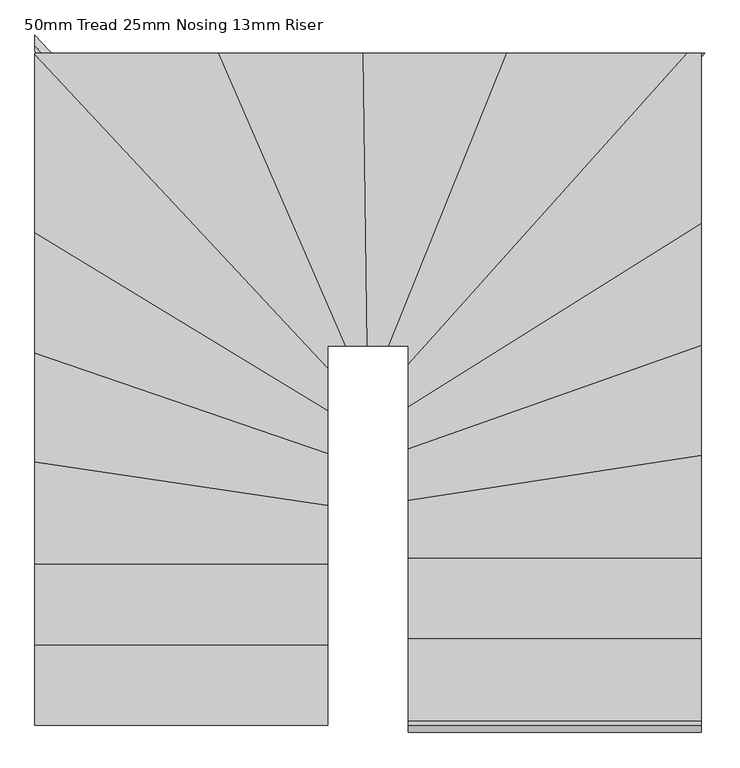
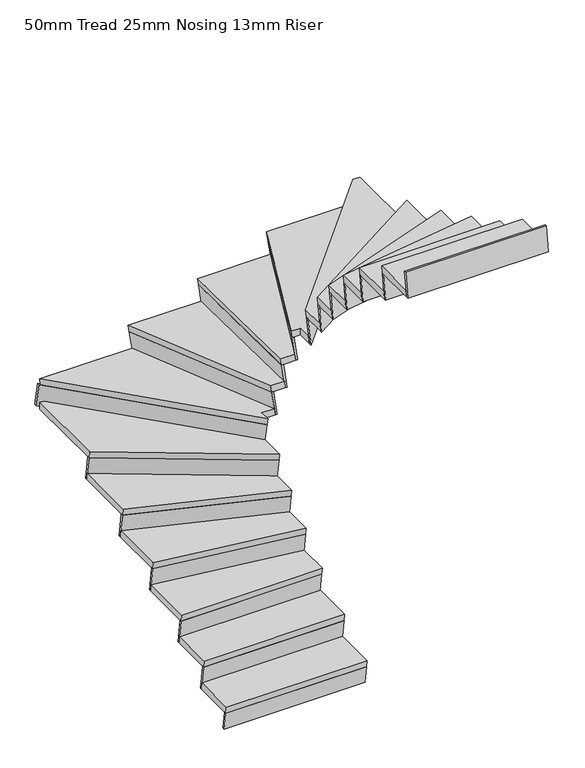
"""IFC4 building model written with IfcOpenShell, lengths in millimetres: stair flight geometry, 50mm Tread 25mm Nosing 13mm Riser."""

from ifc_helpers import new_model, si_unit, origin, place, context, project, spatial, faceted_brep, source, transform, mapped, element, save


def stair_flight_50mm_tread_25mm_nosing_13mm_riser_620a4597(model_context):
    return source(origin(), model_context, "Body", "Brep", [
        faceted_brep([(10289.7497541, -1105.5848061, 3227.2941176), (10289.7497541, -1098.6130213, 3177.2941176), (9289.7239729, -1098.6130213, 3177.2941176), (9289.7239729, -1105.5848061, 3227.2941176), (9289.7239729, -1405.5848061, 3227.2941176), (10289.7497541, -1405.5848061, 3227.2941176), (10289.7497541, -1398.6130213, 3177.2941176), (9289.7239729, -1398.6130213, 3177.2941176)], [[[0, 1, 2, 3]], [[3, 4, 5, 0]], [[2, 1, 6, 7]], [[4, 3, 2, 7]], [[0, 5, 6, 1]], [[5, 4, 7, 6]]]),
        faceted_brep([(10289.7497541, -1398.6130213, 3177.2941176), (10289.7497541, -1380.5848061, 3048.0), (10289.7497541, -1367.9638766, 3048.0), (10289.7497541, -1385.9920918, 3177.2941176), (9289.7239729, -1398.6130213, 3177.2941176), (9289.7239729, -1385.9920918, 3177.2941176), (9289.7239729, -1367.9638766, 3048.0), (9289.7239729, -1380.5848061, 3048.0)], [[[0, 1, 2, 3]], [[4, 5, 6, 7]], [[1, 0, 4, 7]], [[2, 1, 7, 6]], [[3, 2, 6, 5]], [[0, 3, 5, 4]]]),
        faceted_brep([(10289.7497541, -1123.6130213, 3356.5882353), (10289.7497541, -1098.6130213, 3177.2941176), (10289.7497541, -1085.9920918, 3177.2941176), (10289.7497541, -1110.9920918, 3356.5882353), (9289.7239729, -1123.6130213, 3356.5882353), (9289.7239729, -1110.9920918, 3356.5882353), (9289.7239729, -1085.9920918, 3177.2941176), (9289.7239729, -1098.6130213, 3177.2941176)], [[[0, 1, 2, 3]], [[4, 5, 6, 7]], [[1, 0, 4, 7]], [[2, 1, 7, 6]], [[3, 2, 6, 5]], [[0, 3, 5, 4]]]),
        faceted_brep([(9289.7239729, -830.5848061, 3406.5882353), (9289.7239729, -1130.5848061, 3406.5882353), (10289.7497541, -1130.5848061, 3406.5882353), (10289.7497541, -830.5848061, 3406.5882353), (9289.7239729, -823.6130213, 3356.5882353), (10289.7497541, -823.6130213, 3356.5882353), (10289.7497541, -1123.6130213, 3356.5882353), (9289.7239729, -1123.6130213, 3356.5882353)], [[[0, 1, 2, 3]], [[4, 5, 6, 7]], [[1, 0, 4, 7]], [[3, 2, 6, 5]], [[3, 5, 4, 0]], [[2, 1, 7, 6]]]),
        faceted_brep([(10289.7497541, -848.6130213, 3535.8823529), (10289.7497541, -823.6130213, 3356.5882353), (10289.7497541, -810.9920918, 3356.5882353), (10289.7497541, -835.9920918, 3535.8823529), (9289.7239729, -848.6130213, 3535.8823529), (9289.7239729, -835.9920918, 3535.8823529), (9289.7239729, -810.9920918, 3356.5882353), (9289.7239729, -823.6130213, 3356.5882353)], [[[0, 1, 2, 3]], [[4, 5, 6, 7]], [[1, 0, 4, 7]], [[2, 1, 7, 6]], [[3, 2, 6, 5]], [[0, 3, 5, 4]]]),
        faceted_brep([(9289.7239729, -480.7581684, 3585.8823529), (9289.7239729, -855.5848061, 3585.8823529), (10289.7497541, -855.5848061, 3585.8823529), (10289.7497541, -629.8587526, 3585.8823529), (9289.7239729, -473.7093187, 3535.8823529), (10289.7497541, -622.8099029, 3535.8823529), (10289.7497541, -848.6130213, 3535.8823529), (9289.7239729, -848.6130213, 3535.8823529)], [[[0, 1, 2, 3]], [[4, 5, 6, 7]], [[1, 0, 4, 7]], [[3, 2, 6, 5]], [[3, 5, 4, 0]], [[2, 1, 7, 6]]]),
        faceted_brep([(10289.7497541, -648.0862485, 3715.1764706), (10289.7497541, -622.8099029, 3535.8823529), (10289.7497541, -610.0494638, 3535.8823529), (10289.7497541, -635.3258095, 3715.1764706), (9289.7239729, -498.9856643, 3715.1764706), (9289.7239729, -486.2252253, 3715.1764706), (9289.7239729, -460.9488796, 3535.8823529), (9289.7239729, -473.7093187, 3535.8823529)], [[[0, 1, 2, 3]], [[4, 5, 6, 7]], [[1, 0, 4, 7]], [[2, 1, 7, 6]], [[3, 2, 6, 5]], [[0, 3, 5, 4]]]),
        faceted_brep([(9289.7239729, -107.774321, 3765.1764706), (9289.7239729, -506.034514, 3765.1764706), (10289.7497541, -655.1350982, 3765.1764706), (10289.7497541, -450.5397782, 3765.1764706), (9289.7239729, -100.4043758, 3715.1764706), (10289.7497541, -443.169833, 3715.1764706), (10289.7497541, -648.0862485, 3715.1764706), (9289.7239729, -498.9856643, 3715.1764706)], [[[0, 1, 2, 3]], [[4, 5, 6, 7]], [[1, 0, 4, 7]], [[3, 2, 6, 5]], [[3, 5, 4, 0]], [[2, 1, 7, 6]]]),
        faceted_brep([(10289.7497541, -469.5975895, 3894.4705882), (10289.7497541, -443.169833, 3715.1764706), (10289.7497541, -429.8281189, 3715.1764706), (10289.7497541, -456.2558754, 3894.4705882), (9289.7239729, -126.8321323, 3894.4705882), (9289.7239729, -113.4904182, 3894.4705882), (9289.7239729, -87.0626618, 3715.1764706), (9289.7239729, -100.4043758, 3715.1764706)], [[[0, 1, 2, 3]], [[4, 5, 6, 7]], [[1, 0, 4, 7]], [[2, 1, 7, 6]], [[3, 2, 6, 5]], [[0, 3, 5, 4]]]),
        faceted_brep([(9289.7239729, 306.1026023, 3944.4705882), (9289.7239729, -134.2020775, 3944.4705882), (10289.7497541, -476.9675347, 3944.4705882), (10289.7497541, -301.16869, 3944.4705882), (9289.7239729, 314.2591716, 3894.4705882), (10289.7497541, -293.0121207, 3894.4705882), (10289.7497541, -469.5975895, 3894.4705882), (9289.7239729, -126.8321323, 3894.4705882)], [[[0, 1, 2, 3]], [[4, 5, 6, 7]], [[1, 0, 4, 7]], [[3, 2, 6, 5]], [[3, 5, 4, 0]], [[2, 1, 7, 6]]]),
        faceted_brep([(10289.7497541, -322.2606186, 4073.7647059), (10289.7497541, -293.0121207, 3894.4705882), (10289.7497541, -278.2463915, 3894.4705882), (10289.7497541, -307.4948894, 4073.7647059), (9289.7239729, 285.0106737, 4073.7647059), (9289.7239729, 299.7764029, 4073.7647059), (9289.7239729, 329.0249008, 3894.4705882), (9289.7239729, 314.2591716, 3894.4705882)], [[[0, 1, 2, 3]], [[4, 5, 6, 7]], [[1, 0, 4, 7]], [[2, 1, 7, 6]], [[3, 2, 6, 5]], [[0, 3, 5, 4]]]),
        faceted_brep([(9320.7227269, 889.7143644, 4123.7647059), (9289.7239729, 889.7143644, 4123.7647059), (9289.7239729, 276.8541044, 4123.7647059), (10289.7497541, -330.4171879, 4123.7647059), (10289.7497541, -148.9817857, 4123.7647059), (9330.2573955, 889.7143644, 4073.7647059), (10289.7497541, -138.761613, 4073.7647059), (10289.7497541, -322.2606186, 4073.7647059), (9289.7239729, 285.0106737, 4073.7647059), (9289.7239729, 889.7143644, 4073.7647059)], [[[0, 1, 2, 3, 4]], [[5, 6, 7, 8, 9]], [[1, 0, 5, 9]], [[4, 3, 7, 6]], [[4, 6, 5, 0]], [[3, 2, 8, 7]], [[2, 1, 9, 8]]]),
        faceted_brep([(10289.7497541, -175.4099498, 4253.0588235), (10289.7497541, -138.761613, 4073.7647059), (10289.7497541, -120.2601701, 4073.7647059), (10289.7497541, -156.9085068, 4253.0588235), (9289.7239729, 896.5136394, 4253.0588235), (9289.7239729, 915.0150824, 4253.0588235), (9289.7239729, 951.6634191, 4073.7647059), (9289.7239729, 933.1619761, 4073.7647059)], [[[0, 1, 2, 3]], [[4, 5, 6, 7]], [[1, 0, 4, 7]], [[2, 1, 7, 6]], [[3, 2, 6, 5]], [[0, 3, 5, 4]]]),
        faceted_brep([(9944.3142793, 889.7143644, 4303.0588235), (9289.7239729, 889.7143644, 4303.0588235), (9289.7239729, 886.2934667, 4303.0588235), (10289.7497541, -185.6301224, 4303.0588235), (10289.7497541, -110.3114169, 4303.0588235), (10378.5813525, -110.3114169, 4303.0588235), (9951.9150537, 889.7143644, 4253.0588235), (10386.182127, -110.3114169, 4253.0588235), (10289.7497541, -110.3114169, 4253.0588235), (10289.7497541, -175.4099498, 4253.0588235), (9296.0671958, 889.7143644, 4253.0588235), (9289.7239729, 889.7143644, 4286.3228165)], [[[0, 1, 2, 3, 4, 5]], [[6, 7, 8, 9, 10]], [[1, 0, 6, 10, 11]], [[2, 1, 11]], [[4, 3, 9, 8]], [[5, 4, 8, 7]], [[5, 7, 6, 0]], [[3, 2, 11, 10, 9]]]),
        faceted_brep([(10358.9266439, -110.3114169, 4432.3529412), (10386.182127, -110.3114169, 4253.0588235), (10399.9417081, -110.3114169, 4253.0588235), (10372.6862251, -110.3114169, 4432.3529412), (9924.6595707, 889.7143644, 4432.3529412), (9938.4191519, 889.7143644, 4432.3529412), (9965.6746349, 889.7143644, 4253.0588235), (9951.9150537, 889.7143644, 4253.0588235)], [[[0, 1, 2, 3]], [[4, 5, 6, 7]], [[1, 0, 4, 7]], [[2, 1, 7, 6]], [[3, 2, 6, 5]], [[0, 3, 5, 4]]]),
        faceted_brep([(10435.8300538, 889.7143644, 4482.3529412), (9917.0587962, 889.7143644, 4482.3529412), (10351.3258695, -110.3114169, 4482.3529412), (10449.7733926, -110.3114169, 4482.3529412), (10442.8025162, 889.7143644, 4432.3529412), (10456.745855, -110.3114169, 4432.3529412), (10358.9266439, -110.3114169, 4432.3529412), (9924.6595707, 889.7143644, 4432.3529412)], [[[0, 1, 2, 3]], [[4, 5, 6, 7]], [[1, 0, 4, 7]], [[3, 2, 6, 5]], [[3, 5, 4, 0]], [[2, 1, 7, 6]]]),
        faceted_brep([(10431.7434251, -110.3114169, 4611.6470588), (10456.745855, -110.3114169, 4432.3529412), (10469.3680113, -110.3114169, 4432.3529412), (10444.3655813, -110.3114169, 4611.6470588), (10417.8000863, 889.7143644, 4611.6470588), (10430.4222425, 889.7143644, 4611.6470588), (10455.4246725, 889.7143644, 4432.3529412), (10442.8025162, 889.7143644, 4432.3529412)], [[[0, 1, 2, 3]], [[4, 5, 6, 7]], [[1, 0, 4, 7]], [[2, 1, 7, 6]], [[3, 2, 6, 5]], [[0, 3, 5, 4]]]),
        faceted_brep([(10928.1794575, 889.7143644, 4661.6470588), (10410.8276238, 889.7143644, 4661.6470588), (10424.7709627, -110.3114169, 4661.6470588), (10523.7381228, -110.3114169, 4661.6470588), (10935.699827, 889.7143644, 4611.6470588), (10531.2584922, -110.3114169, 4611.6470588), (10431.7434251, -110.3114169, 4611.6470588), (10417.8000863, 889.7143644, 4611.6470588)], [[[0, 1, 2, 3]], [[4, 5, 6, 7]], [[1, 0, 4, 7]], [[3, 2, 6, 5]], [[3, 5, 4, 0]], [[2, 1, 7, 6]]]),
        faceted_brep([(10504.2913321, -110.3114169, 4790.9411765), (10531.2584922, -110.3114169, 4611.6470588), (10544.8725173, -110.3114169, 4611.6470588), (10517.9053572, -110.3114169, 4790.9411765), (10908.7326669, 889.7143644, 4790.9411765), (10922.346692, 889.7143644, 4790.9411765), (10949.3138521, 889.7143644, 4611.6470588), (10935.699827, 889.7143644, 4611.6470588)], [[[0, 1, 2, 3]], [[4, 5, 6, 7]], [[1, 0, 4, 7]], [[2, 1, 7, 6]], [[3, 2, 6, 5]], [[0, 3, 5, 4]]]),
        faceted_brep([(11550.6912543, 889.7143644, 4840.9411765), (10901.2122974, 889.7143644, 4840.9411765), (10496.7709627, -110.3114169, 4840.9411765), (10564.7497541, -110.3114169, 4840.9411765), (10564.7497541, -211.248652, 4840.9411765), (11560.0499961, 889.7143644, 4790.9411765), (10564.7497541, -221.6991996, 4790.9411765), (10564.7497541, -110.3114169, 4790.9411765), (10504.2913321, -110.3114169, 4790.9411765), (10908.7326669, 889.7143644, 4790.9411765)], [[[0, 1, 2, 3, 4]], [[5, 6, 7, 8, 9]], [[1, 0, 5, 9]], [[3, 2, 8, 7]], [[4, 3, 7, 6]], [[4, 6, 5, 0]], [[2, 1, 9, 8]]]),
        faceted_brep([(10564.7497541, -184.2247655, 4970.2352941), (10564.7497541, -221.6991996, 4790.9411765), (10564.7497541, -240.6176872, 4790.9411765), (10564.7497541, -203.1432531, 4970.2352941), (11526.4906492, 889.7143644, 4970.2352941), (11543.4326552, 889.7143644, 4970.2352941), (11576.9920021, 889.7143644, 4790.9411765), (11560.0499961, 889.7143644, 4790.9411765)], [[[0, 1, 2, 3]], [[4, 5, 6, 7]], [[1, 0, 4, 7]], [[2, 1, 7, 6]], [[3, 2, 6, 5]], [[0, 3, 5, 4]]]),
        faceted_brep([(11564.7755354, 278.4528718, 5020.2352941), (11564.7755354, 889.7143644, 5020.2352941), (11517.1319075, 889.7143644, 5020.2352941), (10564.7497541, -173.7742179, 5020.2352941), (10564.7497541, -348.5530054, 5020.2352941), (11564.7755354, 270.2240506, 4970.2352941), (10564.7497541, -356.7818266, 4970.2352941), (10564.7497541, -184.2247655, 4970.2352941), (11526.4906492, 889.7143644, 4970.2352941), (11564.7755354, 889.7143644, 4970.2352941)], [[[0, 1, 2, 3, 4]], [[5, 6, 7, 8, 9]], [[1, 0, 5, 9]], [[2, 1, 9, 8]], [[4, 3, 7, 6]], [[4, 6, 5, 0]], [[3, 2, 8, 7]]]),
        faceted_brep([(10564.7497541, -327.2742418, 5149.5294118), (10564.7497541, -356.7818266, 4970.2352941), (10564.7497541, -371.6783525, 4970.2352941), (10564.7497541, -342.1707677, 5149.5294118), (11564.7755354, 299.7316354, 5149.5294118), (11564.7755354, 284.8351095, 5149.5294118), (11564.7755354, 255.3275247, 4970.2352941), (11564.7755354, 270.2240506, 4970.2352941)], [[[0, 1, 2, 3]], [[4, 5, 6, 7]], [[1, 0, 4, 7]], [[2, 1, 7, 6]], [[3, 2, 6, 5]], [[0, 3, 5, 4]]]),
        faceted_brep([(11564.7755354, -136.4321631, 5199.5294118), (11564.7755354, 307.9604567, 5199.5294118), (10564.7497541, -319.0454205, 5199.5294118), (10564.7497541, -489.6437867, 5199.5294118), (11564.7755354, -143.8260425, 5149.5294118), (10564.7497541, -497.0376661, 5149.5294118), (10564.7497541, -327.2742418, 5149.5294118), (11564.7755354, 299.7316354, 5149.5294118)], [[[0, 1, 2, 3]], [[4, 5, 6, 7]], [[1, 0, 4, 7]], [[3, 2, 6, 5]], [[3, 5, 4, 0]], [[2, 1, 7, 6]]]),
        faceted_brep([(10564.7497541, -470.5240844, 5328.8235294), (10564.7497541, -497.0376661, 5149.5294118), (10564.7497541, -510.4227078, 5149.5294118), (10564.7497541, -483.9091262, 5328.8235294), (11564.7755354, -117.3124608, 5328.8235294), (11564.7755354, -130.6975026, 5328.8235294), (11564.7755354, -157.2110842, 5149.5294118), (11564.7755354, -143.8260425, 5149.5294118)], [[[0, 1, 2, 3]], [[4, 5, 6, 7]], [[1, 0, 4, 7]], [[2, 1, 7, 6]], [[3, 2, 6, 5]], [[0, 3, 5, 4]]]),
        faceted_brep([(11564.7755354, -509.957846, 5378.8235294), (11564.7755354, -109.9185814, 5378.8235294), (10564.7497541, -463.130205, 5378.8235294), (10564.7497541, -663.6782099, 5378.8235294), (11564.7755354, -517.0115171, 5328.8235294), (10564.7497541, -670.731881, 5328.8235294), (10564.7497541, -470.5240844, 5328.8235294), (11564.7755354, -117.3124608, 5328.8235294)], [[[0, 1, 2, 3]], [[4, 5, 6, 7]], [[1, 0, 4, 7]], [[3, 2, 6, 5]], [[3, 5, 4, 0]], [[2, 1, 7, 6]]]),
        faceted_brep([(10564.7497541, -645.4382463, 5508.1176471), (10564.7497541, -670.731881, 5328.8235294), (10564.7497541, -683.5010482, 5328.8235294), (10564.7497541, -658.2074135, 5508.1176471), (11564.7755354, -491.7178824, 5508.1176471), (11564.7755354, -504.4870496, 5508.1176471), (11564.7755354, -529.7806843, 5328.8235294), (11564.7755354, -517.0115171, 5328.8235294)], [[[0, 1, 2, 3]], [[4, 5, 6, 7]], [[1, 0, 4, 7]], [[2, 1, 7, 6]], [[3, 2, 6, 5]], [[0, 3, 5, 4]]]),
        faceted_brep([(11564.7755354, -861.5243932, 5558.1176471), (11564.7755354, -484.6642113, 5558.1176471), (10564.7497541, -638.3845752, 5558.1176471), (10564.7497541, -861.5243932, 5558.1176471), (11564.7755354, -868.496178, 5508.1176471), (10564.7497541, -868.496178, 5508.1176471), (10564.7497541, -645.4382463, 5508.1176471), (11564.7755354, -491.7178824, 5508.1176471)], [[[0, 1, 2, 3]], [[4, 5, 6, 7]], [[1, 0, 4, 7]], [[3, 2, 6, 5]], [[3, 5, 4, 0]], [[2, 1, 7, 6]]]),
        faceted_brep([(10564.7497541, -843.496178, 5687.4117647), (10564.7497541, -868.496178, 5508.1176471), (10564.7497541, -881.1171075, 5508.1176471), (10564.7497541, -856.1171075, 5687.4117647), (11564.7755354, -843.496178, 5687.4117647), (11564.7755354, -856.1171075, 5687.4117647), (11564.7755354, -881.1171075, 5508.1176471), (11564.7755354, -868.496178, 5508.1176471)], [[[0, 1, 2, 3]], [[4, 5, 6, 7]], [[1, 0, 4, 7]], [[2, 1, 7, 6]], [[3, 2, 6, 5]], [[0, 3, 5, 4]]]),
        faceted_brep([(11564.7755354, -1136.5243932, 5737.4117647), (11564.7755354, -836.5243932, 5737.4117647), (10564.7497541, -836.5243932, 5737.4117647), (10564.7497541, -1136.5243932, 5737.4117647), (11564.7755354, -1143.496178, 5687.4117647), (10564.7497541, -1143.496178, 5687.4117647), (10564.7497541, -843.496178, 5687.4117647), (11564.7755354, -843.496178, 5687.4117647)], [[[0, 1, 2, 3]], [[4, 5, 6, 7]], [[1, 0, 4, 7]], [[3, 2, 6, 5]], [[3, 5, 4, 0]], [[2, 1, 7, 6]]]),
        faceted_brep([(10564.7497541, -1118.496178, 5866.7058824), (10564.7497541, -1143.496178, 5687.4117647), (10564.7497541, -1156.1171075, 5687.4117647), (10564.7497541, -1131.1171075, 5866.7058824), (11564.7755354, -1118.496178, 5866.7058824), (11564.7755354, -1131.1171075, 5866.7058824), (11564.7755354, -1156.1171075, 5687.4117647), (11564.7755354, -1143.496178, 5687.4117647)], [[[0, 1, 2, 3]], [[4, 5, 6, 7]], [[1, 0, 4, 7]], [[2, 1, 7, 6]], [[3, 2, 6, 5]], [[0, 3, 5, 4]]]),
        faceted_brep([(10564.7497541, -1393.496178, 6046.0), (10564.7497541, -1418.496178, 5866.7058824), (10564.7497541, -1431.1171075, 5866.7058824), (10564.7497541, -1406.1171075, 6046.0), (11564.7755354, -1393.496178, 6046.0), (11564.7755354, -1406.1171075, 6046.0), (11564.7755354, -1431.1171075, 5866.7058824), (11564.7755354, -1418.496178, 5866.7058824)], [[[0, 1, 2, 3]], [[4, 5, 6, 7]], [[1, 0, 4, 7]], [[2, 1, 7, 6]], [[3, 2, 6, 5]], [[0, 3, 5, 4]]]),
        faceted_brep([(11564.7755354, -1411.5243932, 5916.7058824), (11564.7755354, -1111.5243932, 5916.7058824), (10564.7497541, -1111.5243932, 5916.7058824), (10564.7497541, -1411.5243932, 5916.7058824), (11564.7755354, -1418.496178, 5866.7058824), (10564.7497541, -1418.496178, 5866.7058824), (10564.7497541, -1118.496178, 5866.7058824), (11564.7755354, -1118.496178, 5866.7058824)], [[[0, 1, 2, 3]], [[4, 5, 6, 7]], [[1, 0, 4, 7]], [[3, 2, 6, 5]], [[3, 5, 4, 0]], [[2, 1, 7, 6]]]),
    ])


if __name__ == "__main__":
    model = new_model("IFC4")
    model_context = context("Model", 3, world=origin())
    ifc_project = project(units=[si_unit("LENGTHUNIT", "METRE", prefix="MILLI")], contexts=[model_context])
    site = spatial("IfcSite", under=ifc_project)
    building = spatial("IfcBuilding", under=site)
    placement = place(None, origin())
    stair_flight_50mm_tread_25mm_nosing_13mm_riser_shape = stair_flight_50mm_tread_25mm_nosing_13mm_riser_620a4597(model_context)
    element("IfcStairFlight", 1, ObjectType="50mm Tread 25mm Nosing 13mm Riser", at=placement, inside=building, context=model_context, shape_type="MappedRepresentation", body=[
        mapped(stair_flight_50mm_tread_25mm_nosing_13mm_riser_shape, transform((0.0, 0.0, 0.0), x_axis=(1.0, 0.0, 0.0), y_axis=(0.0, 1.0, 0.0), z_axis=(0.0, 0.0, 1.0))),
    ])
    save(model, "model.ifc")
